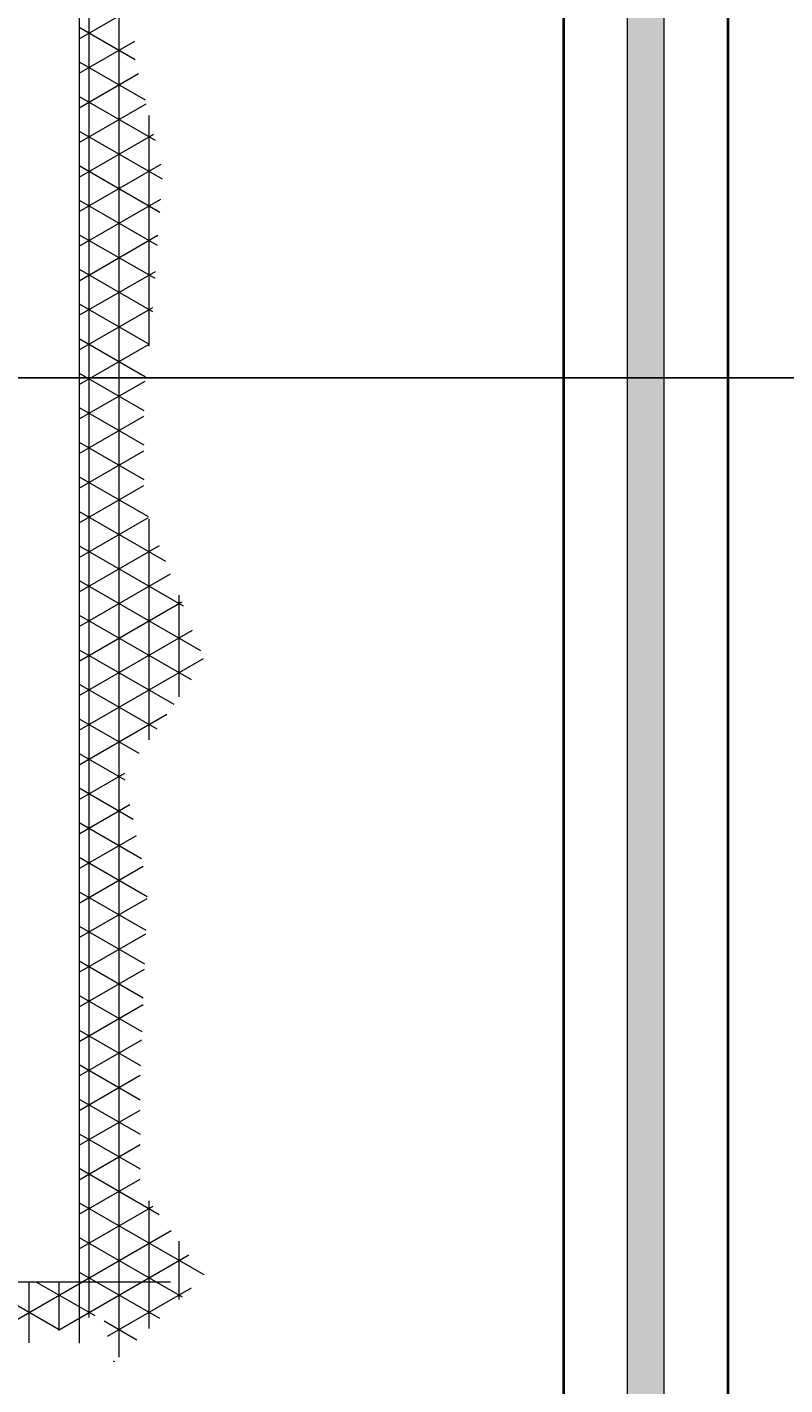
# Model space of a CAD drawing. Units: inches. Extents: x 2330 to 3943, y 1763 to 3461.
# Tile 35 of 40: x 3417 to 3459, y 3024 to 3098. Entities that reach past the tile are written whole.
import ezdxf

# ---------------------------------------------------------------- set-up
doc = ezdxf.new("R2010")
doc.units = ezdxf.units.IN
for name, color, linetype, lineweight in [('A-ANNO-DIMS', 2, 'Continuous', 18), ('A-FURN', 8, 'Continuous', 13), ('A-GLAZ', 4, 'Continuous', 18), ('A-WALL', 7, 'Continuous', 40)]:
    doc.layers.add(name, color=color, linetype=linetype, lineweight=lineweight)
doc.styles.get("Standard").update_dxf_attribs({"font": 'arial.ttf'})
doc.dimstyles.get("Standard").update_dxf_attribs({"dimtxt": 0.18, "dimasz": 0.18, "dimexe": 0.18, "dimexo": 0.0625, "dimgap": 0.09, "dimtad": 0, "dimtih": 1, "dimtoh": 1, "dimdec": 4, "dimzin": 0, "dimdsep": 46, "dimtxsty": 'Standard', "dimcen": 0.09, "dimadec": 0, "dimazin": 0, "dimtfac": 1, "dimtdec": 4, "dimtofl": 0, "dimtmove": 0, "dimatfit": 3, "dimfxl": 1, "dimtolj": 1, "dimtzin": 0, "dimarcsym": 0})

# ---------------------------------------------------------------- blocks, each defined once
blk = doc.blocks.new('A$C200C7901')
for p, q in [((2.3121, 1.6596), (2.3121, 0.0201)), ((2.4073, 0.0839), (0.9625, 0.0839))]:
    blk.add_line(p, q)
at = {"linetype": 'ByBlock'}
for p, q in [((2.3224, 0.0468), (2.3224, 1.6627)), ((2.3224, 0.0468), (2.3224, 1.6627)), ((2.3537, 0.0056), (2.3537, 1.634)), ((2.3537, 0.0056), (2.3537, 1.634)), ((2.3121, 1.3815), (2.3848, 1.4235)), ((2.3121, 1.3815), (2.3848, 1.4235)), ((2.3121, 1.3934), (2.3703, 1.3598)), ((2.3121, 1.3934), (2.3703, 1.3598)), ((2.3121, 1.3454), (2.37, 1.3788)), ((2.3121, 1.3454), (2.37, 1.3788)), ((2.3121, 1.3573), (2.3808, 1.3176)), ((2.3121, 1.3573), (2.3808, 1.3176)), ((2.3121, 1.3093), (2.374, 1.345)), ((2.3121, 1.3093), (2.374, 1.345)), ((2.3121, 1.3212), (2.3914, 1.2754)), ((2.3121, 1.3212), (2.3914, 1.2754)), ((2.3121, 1.2732), (2.3819, 1.3135)), ((2.3121, 1.2732), (2.3819, 1.3135)), ((2.3849, 1.0607), (2.3849, 1.3013)), ((2.3849, 1.0607), (2.3849, 1.3013)), ((2.3121, 1.2851), (2.3985, 1.2352)), ((2.3121, 1.2851), (2.3985, 1.2352)), ((2.3121, 1.2371), (2.3898, 1.282)), ((2.3121, 1.2371), (2.3898, 1.282)), ((2.3121, 1.2011), (2.3976, 1.2504)), ((2.3121, 1.2011), (2.3976, 1.2504)), ((2.3121, 1.249), (2.396, 1.2006)), ((2.3121, 1.249), (2.396, 1.2006)), ((2.3121, 1.165), (2.397, 1.214)), ((2.3121, 1.165), (2.397, 1.214)), ((2.3121, 1.2129), (2.3935, 1.166)), ((2.3121, 1.2129), (2.3935, 1.166)), ((2.3121, 1.1768), (2.3909, 1.1314)), ((2.3121, 1.1768), (2.3909, 1.1314)), ((2.3121, 1.1289), (2.3942, 1.1763)), ((2.3121, 1.1289), (2.3942, 1.1763)), ((2.3121, 1.1408), (2.3884, 1.0967)), ((2.3121, 1.1408), (2.3884, 1.0967)), ((2.3121, 1.0928), (2.3915, 1.1386)), ((2.3121, 1.0928), (2.3915, 1.1386)), ((2.3121, 1.1047), (2.3851, 1.0625)), ((2.3121, 1.1047), (2.3851, 1.0625)), ((2.3121, 1.0567), (2.3887, 1.1009)), ((2.3121, 1.0567), (2.3887, 1.1009)), ((2.3121, 1.0686), (2.3813, 1.0286)), ((2.3121, 1.0686), (2.3813, 1.0286)), ((2.3121, 1.0206), (2.3851, 1.0628)), ((2.3121, 1.0206), (2.3851, 1.0628)), ((2.3121, 1.0325), (2.3795, 0.9936)), ((2.3121, 1.0325), (2.3795, 0.9936)), ((2.3121, 0.9846), (2.3809, 1.0242)), ((2.3121, 0.9846), (2.3809, 1.0242)), ((2.3121, 0.9964), (2.3795, 0.9575)), ((2.3121, 0.9964), (2.3795, 0.9575)), ((2.3121, 0.9485), (2.3795, 0.9874)), ((2.3121, 0.9485), (2.3795, 0.9874)), ((2.3121, 0.9603), (2.3795, 0.9215)), ((2.3121, 0.9603), (2.3795, 0.9215)), ((2.3121, 0.9124), (2.3795, 0.9513)), ((2.3121, 0.9124), (2.3795, 0.9513)), ((2.3121, 0.9243), (2.3838, 0.8829)), ((2.3121, 0.9243), (2.3838, 0.8829)), ((2.3121, 0.8763), (2.3795, 0.9152)), ((2.3121, 0.8763), (2.3795, 0.9152)), ((2.3121, 0.8882), (2.4022, 0.8362)), ((2.3121, 0.8882), (2.4022, 0.8362)), ((2.3121, 0.8402), (2.3842, 0.8818)), ((2.3121, 0.8402), (2.3842, 0.8818)), ((2.3849, 0.6497), (2.3849, 0.8801)), ((2.3849, 0.6497), (2.3849, 0.8801)), ((2.3121, 0.8041), (2.3958, 0.8524)), ((2.3121, 0.8041), (2.3958, 0.8524)), ((2.3121, 0.8521), (2.4205, 0.7895)), ((2.3121, 0.8521), (2.4205, 0.7895)), ((2.3121, 0.7681), (2.4073, 0.823)), ((2.3121, 0.7681), (2.4073, 0.823)), ((2.3121, 0.816), (2.4384, 0.7431)), ((2.3121, 0.816), (2.4384, 0.7431)), ((2.3121, 0.732), (2.4189, 0.7936)), ((2.3121, 0.732), (2.4189, 0.7936)), ((2.4162, 0.6946), (2.4162, 0.8006)), ((2.4162, 0.6946), (2.4162, 0.8006)), ((2.3121, 0.7799), (2.4287, 0.7126)), ((2.3121, 0.7799), (2.4287, 0.7126)), ((2.3121, 0.6959), (2.4303, 0.7641)), ((2.3121, 0.6959), (2.4303, 0.7641)), ((2.3121, 0.7438), (2.4108, 0.6869)), ((2.3121, 0.7438), (2.4108, 0.6869)), ((2.3121, 0.6598), (2.4417, 0.7346)), ((2.3121, 0.6598), (2.4417, 0.7346)), ((2.3121, 0.7078), (2.3929, 0.6611)), ((2.3121, 0.7078), (2.3929, 0.6611)), ((2.3121, 0.6237), (2.4036, 0.6765)), ((2.3121, 0.6237), (2.4036, 0.6765)), ((2.3121, 0.6717), (2.3744, 0.6357)), ((2.3121, 0.6717), (2.3744, 0.6357)), ((2.3121, 0.6356), (2.3598, 0.6081)), ((2.3121, 0.6356), (2.3598, 0.6081)), ((2.3121, 0.5876), (2.3598, 0.6151)), ((2.3121, 0.5876), (2.3598, 0.6151)), ((2.3121, 0.5995), (2.3682, 0.5671)), ((2.3121, 0.5995), (2.3682, 0.5671)), ((2.3121, 0.5515), (2.365, 0.5821)), ((2.3121, 0.5515), (2.365, 0.5821)), ((2.3121, 0.5634), (2.3771, 0.5259)), ((2.3121, 0.5634), (2.3771, 0.5259)), ((2.3121, 0.5155), (2.3719, 0.55)), ((2.3121, 0.5155), (2.3719, 0.55)), ((2.3121, 0.5273), (2.383, 0.4864)), ((2.3121, 0.5273), (2.383, 0.4864)), ((2.3121, 0.4794), (2.3788, 0.5179)), ((2.3121, 0.4794), (2.3788, 0.5179)), ((2.3121, 0.4912), (2.3817, 0.4511)), ((2.3121, 0.4912), (2.3817, 0.4511)), ((2.3121, 0.4433), (2.383, 0.4842)), ((2.3121, 0.4433), (2.383, 0.4842)), ((2.3121, 0.4552), (2.3803, 0.4158)), ((2.3121, 0.4552), (2.3803, 0.4158)), ((2.3121, 0.4072), (2.3815, 0.4473)), ((2.3121, 0.4072), (2.3815, 0.4473)), ((2.3121, 0.4191), (2.3789, 0.3805)), ((2.3121, 0.4191), (2.3789, 0.3805)), ((2.3121, 0.3711), (2.3801, 0.4103)), ((2.3121, 0.3711), (2.3801, 0.4103)), ((2.3121, 0.383), (2.3775, 0.3452)), ((2.3121, 0.383), (2.3775, 0.3452)), ((2.3121, 0.335), (2.3786, 0.3734)), ((2.3121, 0.335), (2.3786, 0.3734)), ((2.3121, 0.3469), (2.3761, 0.31)), ((2.3121, 0.3469), (2.3761, 0.31)), ((2.3121, 0.299), (2.3772, 0.3365)), ((2.3121, 0.299), (2.3772, 0.3365)), ((2.3121, 0.3108), (2.3755, 0.2742)), ((2.3121, 0.3108), (2.3755, 0.2742)), ((2.3121, 0.2629), (2.3757, 0.2996)), ((2.3121, 0.2629), (2.3757, 0.2996)), ((2.3121, 0.2747), (2.3755, 0.2381)), ((2.3121, 0.2747), (2.3755, 0.2381)), ((2.3121, 0.2268), (2.3755, 0.2634)), ((2.3121, 0.2268), (2.3755, 0.2634)), ((2.3121, 0.2387), (2.3755, 0.202)), ((2.3121, 0.2387), (2.3755, 0.202)), ((2.3121, 0.1907), (2.3755, 0.2273)), ((2.3121, 0.1907), (2.3755, 0.2273)), ((2.3121, 0.2026), (2.3953, 0.1545)), ((2.3121, 0.2026), (2.3953, 0.1545)), ((2.3121, 0.1546), (2.3755, 0.1912)), ((2.3121, 0.1546), (2.3755, 0.1912)), ((2.3121, 0.1665), (2.4419, 0.0916)), ((2.3121, 0.1665), (2.4419, 0.0916)), ((2.3121, 0.1185), (2.3891, 0.163)), ((2.3121, 0.1185), (2.3891, 0.163)), ((2.3849, 0.0355), (2.3849, 0.1686)), ((2.3849, 0.0355), (2.3849, 0.1686)), ((2.2208, 0.0297), (2.4078, 0.1377)), ((2.2208, 0.0297), (2.4078, 0.1377)), ((2.3121, 0.1304), (2.4193, 0.0685)), ((2.3121, 0.1304), (2.4193, 0.0685)), ((2.4162, 0.0655), (2.4162, 0.1264)), ((2.4162, 0.0655), (2.4162, 0.1264)), ((2.2903, 0.0337), (2.4265, 0.1124)), ((2.2903, 0.0337), (2.4265, 0.1124)), ((2.3121, 0.0943), (2.3958, 0.046)), ((2.3121, 0.0943), (2.3958, 0.046)), ((2.2051, 0.0839), (2.2913, 0.0342)), ((2.2051, 0.0839), (2.2913, 0.0342)), ((2.2599, 0.0205), (2.2599, 0.0839)), ((2.2599, 0.0205), (2.2599, 0.0839)), ((2.2676, 0.0839), (2.3285, 0.0488)), ((2.2676, 0.0839), (2.3285, 0.0488)), ((2.2912, 0.0341), (2.2912, 0.0839)), ((2.2912, 0.0341), (2.2912, 0.0839)), ((2.3417, 0.0273), (2.429, 0.0777)), ((2.3417, 0.0273), (2.429, 0.0777)), ((2.338, 0.0433), (2.3723, 0.0235)), ((2.338, 0.0433), (2.3723, 0.0235)), ((2.3476, 0.0017), (2.3488, 0.001)), ((2.3476, 0.0017), (2.3488, 0.001))]:
    blk.add_line(p, q, dxfattribs=at)
blk = doc.blocks.new('WINDOW-96IN')
h = blk.add_hatch(color=256)
h.dxf.hatch_style = 1
h.paths.add_polyline_path([(5.5, 96), (3.5, 96), (3.5, 0), (5.5, 0)])
for p, q in [((3.5, 96), (3.5, 0)), ((5.5, 96), (5.5, 0))]:
    blk.add_line(p, q)
blk = doc.blocks.new('*D86')
at = {"layer": 'A-ANNO-DIMS', "color": 0, "lineweight": -2, "transparency": 16777216}
for p, q in [((2979.184, 3100.039), (3942.541, 3100.039)), ((3942.361, 3099.859), (3942.361, 3089.719)), ((3942.361, 3079.219), (3942.361, 3089.358)), ((2979.184, 3079.039), (3942.541, 3079.039))]:
    blk.add_line(p, q, dxfattribs=at)
at = {"layer": 'A-ANNO-DIMS', "color": 0, "transparency": 16777216}
for points in [[(3942.331, 3099.859), (3942.391, 3099.859), (3942.361, 3100.039)], [(3942.331, 3079.219), (3942.391, 3079.219), (3942.361, 3079.039)]]:
    blk.add_solid(points, dxfattribs=at)
at = {"layer": 'Defpoints', "color": 0, "transparency": 16777216}
for p in [(2979.122, 3100.039), (2979.122, 3079.039), (3942.361, 3079.039)]:
    blk.add_point(p, dxfattribs=at)
at = {"layer": 'A-ANNO-DIMS', "color": 0, "transparency": 16777216, "insert": (3942.361, 3089.539), "char_height": 0.18, "attachment_point": 5}
blk.add_mtext('\\A1;21', dxfattribs=at)

msp = doc.modelspace()

# ---------------------------------------------------------------- linework, layer by layer
at = {"layer": 'A-WALL'}
for p, q in [((3455.6605, 3162.6524), (3455.6605, 2970.6524)), ((3446.6605, 3153.6524), (3446.6605, 2979.6524))]:
    msp.add_line(p, q, dxfattribs=at)

# ---------------------------------------------------------------- block references
at = {"layer": 'A-FURN', "xscale": 52.5181391560459, "yscale": 52.5181391560459, "zscale": 52.5181391560459}
msp.add_blockref('A$C200C7901', (3298.7219, 3025.0763), dxfattribs=at)
at = {"layer": 'A-GLAZ'}
msp.add_blockref('WINDOW-96IN', (3446.6605, 3018.6524), dxfattribs=at)

# ---------------------------------------------------------------- dimensions: what is measured, and where the dimension line sits
at = {"layer": 'A-ANNO-DIMS'}
dim = msp.add_linear_dim(base=(3942.361, 3079.0386), p1=(2979.1218, 3100.0386), p2=(2979.1218, 3079.0386), angle=90, dimstyle='Standard', override={"dimdec": 0, "dimlfac": 1, "dimrnd": 0, "dimzin": 0, "dimdsep": 46, "dimlunit": 2}, dxfattribs=at)
dim.commit()
dim.dimension.update_dxf_attribs({"geometry": '*D86', "text_midpoint": (3942.361, 3089.5386)})

doc.saveas('drawing.dxf')
